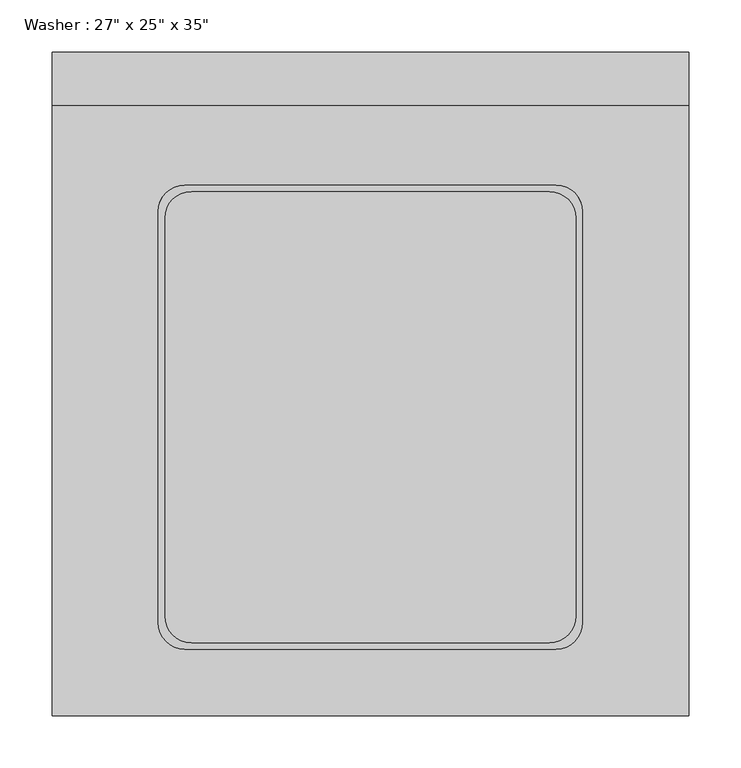
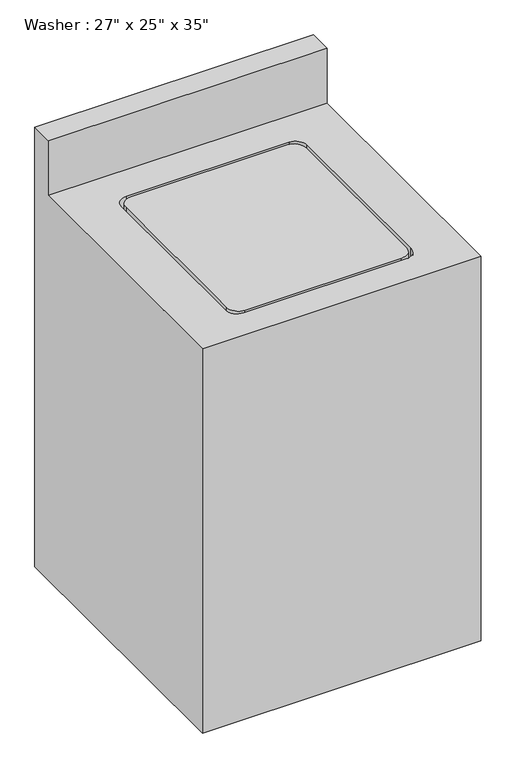
"""IFC4 building model written with IfcOpenShell, lengths in millimetres: proxy geometry."""

from ifc_helpers import new_model, si_unit, point, frame, frame_2d, origin, place, context, project, spatial, polyline, circle_curve, trimmed, segment, composite_curve, outline, extrude, source, transform, mapped, element, save
from ifc_brep_helpers import plane_surface, revolved_surface, advanced_brep


def proxy_67057e99(model_context):
    return source(origin(), model_context, "Body", "SolidModel", [
        extrude(outline(composite_curve([segment(trimmed(circle_curve(frame_2d((210.8674685, 437.8995648)), 25.4), [point((185.4674685, 437.8995648))], [point((210.8674685, 463.2995648))], False, "CARTESIAN"), True, "CONTINUOUS"), segment(polyline([(210.8674685, 463.2995648), (553.7674685, 463.2995648)]), True, "CONTINUOUS"), segment(trimmed(circle_curve(frame_2d((553.7674685, 437.8995648)), 25.4), [point((553.7674685, 463.2995648))], [point((579.1674685, 437.8995648))], False, "CARTESIAN"), True, "CONTINUOUS"), segment(polyline([(579.1674685, 437.8995648), (579.1674685, 56.8995648)]), True, "CONTINUOUS"), segment(trimmed(circle_curve(frame_2d((553.7674685, 56.8995648)), 25.4), [point((579.1674685, 56.8995648))], [point((553.7674685, 31.4995648))], False, "CARTESIAN"), True, "CONTINUOUS"), segment(polyline([(553.7674685, 31.4995648), (210.8674685, 31.4995648)]), True, "CONTINUOUS"), segment(trimmed(circle_curve(frame_2d((210.8674685, 56.8995648)), 25.4), [point((210.8674685, 31.4995648))], [point((185.4674685, 56.8995648))], False, "CARTESIAN"), True, "CONTINUOUS"), segment(polyline([(185.4674685, 56.8995648), (185.4674685, 437.8995648)]), True, "CONTINUOUS")], self_intersect=False)), frame((0.0, 0.0, 863.6), z_axis=(0.0, 0.0, 1.0), x_axis=(1.0, 0.0, 0.0)), (0.0, 0.0, 1.0), 25.4),
        advanced_brep(
        [(77.5174685, 545.8495648, 889.0), (77.5174685, 545.8495648, 1016.0), (77.5174685, 596.6495648, 1016.0), (77.5174685, 596.6495648, 0.0), (77.5174685, -38.3504352, 0.0), (77.5174685, -38.3504352, 889.0), (687.1174685, 596.6495648, 1016.0), (687.1174685, 545.8495648, 1016.0), (687.1174685, 545.8495648, 889.0), (687.1174685, -38.3504352, 889.0), (687.1174685, -38.3504352, 0.0), (687.1174685, 596.6495648, 0.0), (204.5174685, 469.4681955, 889.0), (560.1174685, 469.4681955, 889.0), (585.5174685, 444.0681955, 889.0), (585.5174685, 50.5495648, 889.0), (560.1174685, 25.1495648, 889.0), (204.5174685, 25.1495648, 889.0), (179.1174685, 50.5495648, 889.0), (179.1174685, 444.0681955, 889.0), (560.1174685, 469.4681955, 838.2), (204.5174685, 469.4681955, 838.2), (179.1174685, 444.0681955, 838.2), (179.1174685, 50.5495648, 838.2), (204.5174685, 25.1495648, 838.2), (560.1174685, 25.1495648, 838.2), (585.5174685, 50.5495648, 838.2), (585.5174685, 444.0681955, 838.2)],
        [
            (0, 1),
            (1, 2),
            (2, 3),
            (3, 4),
            (4, 5),
            (5, 0),
            (6, 7),
            (7, 8),
            (8, 9),
            (9, 10),
            (10, 11),
            (11, 6),
            (0, 8),
            (7, 1),
            (6, 2),
            (11, 3),
            (5, 9),
            (12, 13),
            (13, 14, circle_curve(frame((560.1174685, 444.0681955, 889.0), z_axis=(0.0, 0.0, -1.0), x_axis=(0.0, -1.0, 0.0)), 25.4)),
            (14, 15),
            (15, 16, circle_curve(frame((560.1174685, 50.5495648, 889.0), z_axis=(0.0, 0.0, -1.0), x_axis=(0.0, -1.0, 0.0)), 25.4)),
            (16, 17),
            (17, 18, circle_curve(frame((204.5174685, 50.5495648, 889.0), z_axis=(0.0, 0.0, -1.0), x_axis=(0.0, -1.0, 0.0)), 25.4)),
            (18, 19),
            (19, 12, circle_curve(frame((204.5174685, 444.0681955, 889.0), z_axis=(0.0, 0.0, -1.0), x_axis=(0.0, -1.0, 0.0)), 25.4)),
            (10, 4),
            (20, 21),
            (21, 22, circle_curve(frame((204.5174685, 444.0681955, 838.2), z_axis=(0.0, 0.0, 1.0), x_axis=(0.0, -1.0, 0.0)), 25.4)),
            (22, 23),
            (23, 24, circle_curve(frame((204.5174685, 50.5495648, 838.2), z_axis=(0.0, 0.0, 1.0), x_axis=(0.0, -1.0, 0.0)), 25.4)),
            (24, 25),
            (25, 26, circle_curve(frame((560.1174685, 50.5495648, 838.2), z_axis=(0.0, 0.0, 1.0), x_axis=(0.0, -1.0, 0.0)), 25.4)),
            (26, 27),
            (27, 20, circle_curve(frame((560.1174685, 444.0681955, 838.2), z_axis=(0.0, 0.0, 1.0), x_axis=(0.0, -1.0, 0.0)), 25.4)),
            (20, 13),
            (12, 21),
            (19, 22),
            (18, 23),
            (17, 24),
            (16, 25),
            (15, 26),
            (14, 27),
        ],
        [
            plane_surface(frame((77.5174685, 545.8495648, 889.0), z_axis=(-1.0, 0.0, 0.0), x_axis=(0.0, 0.0, 1.0))),
            plane_surface(frame((687.1174685, 545.8495648, 889.0), z_axis=(1.0, 0.0, 0.0), x_axis=(0.0, 0.0, -1.0))),
            plane_surface(frame((77.5174685, 545.8495648, 889.0), z_axis=(0.0, -1.0, 0.0), x_axis=(1.0, 0.0, 0.0))),
            plane_surface(frame((77.5174685, 545.8495648, 1016.0), z_axis=(0.0, 0.0, 1.0), x_axis=(1.0, 0.0, 0.0))),
            plane_surface(frame((77.5174685, 596.6495648, 1016.0), z_axis=(0.0, 1.0, 0.0), x_axis=(1.0, 0.0, 0.0))),
            plane_surface(frame((77.5174685, -38.3504352, 889.0), z_axis=(0.0, 0.0, 1.0), x_axis=(0.0, -1.0, 0.0))),
            plane_surface(frame((77.5174685, -38.3504352, 0.0), z_axis=(0.0, 0.0, -1.0), x_axis=(0.0, 1.0, 0.0))),
            plane_surface(frame((77.5174685, -38.3504352, 889.0), z_axis=(0.0, -1.0, 0.0), x_axis=(0.0, 0.0, -1.0))),
            plane_surface(frame((204.5174685, 469.4681955, 838.2), z_axis=(0.0, 0.0, 1.0), x_axis=(1.0, 0.0, 0.0))),
            plane_surface(frame((560.1174685, 469.4681955, 889.0), z_axis=(0.0, -1.0, 0.0), x_axis=(0.0, 0.0, -1.0))),
            revolved_surface(polyline([(204.5174685, 418.6681955, 889.0), (204.5174685, 418.6681955, 838.2)]), (204.5174685, 444.0681955, 838.2), (0.0, 0.0, 1.0)),
            plane_surface(frame((179.1174685, 444.0681955, 889.0), z_axis=(1.0, 0.0, 0.0), x_axis=(0.0, 0.0, -1.0))),
            revolved_surface(polyline([(204.5174685, 25.1495648, 889.0), (204.5174685, 25.1495648, 838.2)]), (204.5174685, 50.5495648, 838.2), (0.0, 0.0, 1.0)),
            plane_surface(frame((204.5174685, 25.1495648, 889.0), z_axis=(0.0, 1.0, 0.0), x_axis=(0.0, 0.0, -1.0))),
            revolved_surface(polyline([(560.1174685, 25.1495648, 889.0), (560.1174685, 25.1495648, 838.2)]), (560.1174685, 50.5495648, 838.2), (0.0, 0.0, 1.0)),
            plane_surface(frame((585.5174685, 50.5495648, 889.0), z_axis=(-1.0, 0.0, 0.0), x_axis=(0.0, 0.0, -1.0))),
            revolved_surface(polyline([(560.1174685, 418.6681955, 889.0), (560.1174685, 418.6681955, 838.2)]), (560.1174685, 444.0681955, 838.2), (0.0, 0.0, 1.0)),
        ],
        [
            (0, [[1, 2, 3, 4, 5, 6]]),
            (1, [[7, 8, 9, 10, 11, 12]]),
            (2, [[-1, 13, -8, 14]]),
            (3, [[-2, -14, -7, 15]]),
            (4, [[-15, -12, 16, -3]]),
            (5, [[17, -9, -13, -6], [18, 19, 20, 21, 22, 23, 24, 25]]),
            (6, [[-16, -11, 26, -4]]),
            (7, [[-17, -5, -26, -10]]),
            (8, [[27, 28, 29, 30, 31, 32, 33, 34]]),
            (9, [[-27, 35, -18, 36]]),
            (10, [[-28, -36, -25, 37]]),
            (11, [[-29, -37, -24, 38]]),
            (12, [[-30, -38, -23, 39]]),
            (13, [[-31, -39, -22, 40]]),
            (14, [[-32, -40, -21, 41]]),
            (15, [[-33, -41, -20, 42]]),
            (16, [[-34, -42, -19, -35]]),
        ],
    ),
    ])


if __name__ == "__main__":
    model = new_model("IFC4")
    model_context = context("Model", 3, world=origin())
    ifc_project = project(units=[si_unit("LENGTHUNIT", "METRE", prefix="MILLI")], contexts=[model_context])
    site = spatial("IfcSite", under=ifc_project)
    building = spatial("IfcBuilding", under=site)
    placement = place(None, origin())
    proxy_shape = proxy_67057e99(model_context)
    element("IfcBuildingElementProxy", 1, Name="Washer : 27\" x 25\" x 35\"", ObjectType="Washer : 27\" x 25\" x 35\"", at=placement, inside=building, context=model_context, shape_type="MappedRepresentation", body=[
        mapped(proxy_shape, transform((0.0, 0.0, 0.0), x_axis=(1.0, 0.0, 0.0), y_axis=(0.0, 1.0, 0.0), z_axis=(0.0, 0.0, 1.0))),
    ])
    save(model, "model.ifc")

# Revit data of these elements
# Type "Washer : 27\" x 25\" x 35\""
#   Label = "W"
#   Assembly Code = "E1090400"
#   Depth = 2' - 1"
#   Height = 2' - 11"
#   Width = 2' - 0"
#   Washer Material = Steel, Paint Finish, Ivory, Matte
#   Default Elevation = 0
# Element 1 (IfcBuildingElementProxy, "Washer : 27\" x 25\" x 35\"")
#   Materials on its faces: "Steel, Paint Finish, Ivory, Matte"
# Materials
#   "Steel, Paint Finish, Ivory, Matte": class "Metal", colour RGB 247 247 239, transparency 0, Description = "Steel, paint finish, ivory, matte", Cost = 0
